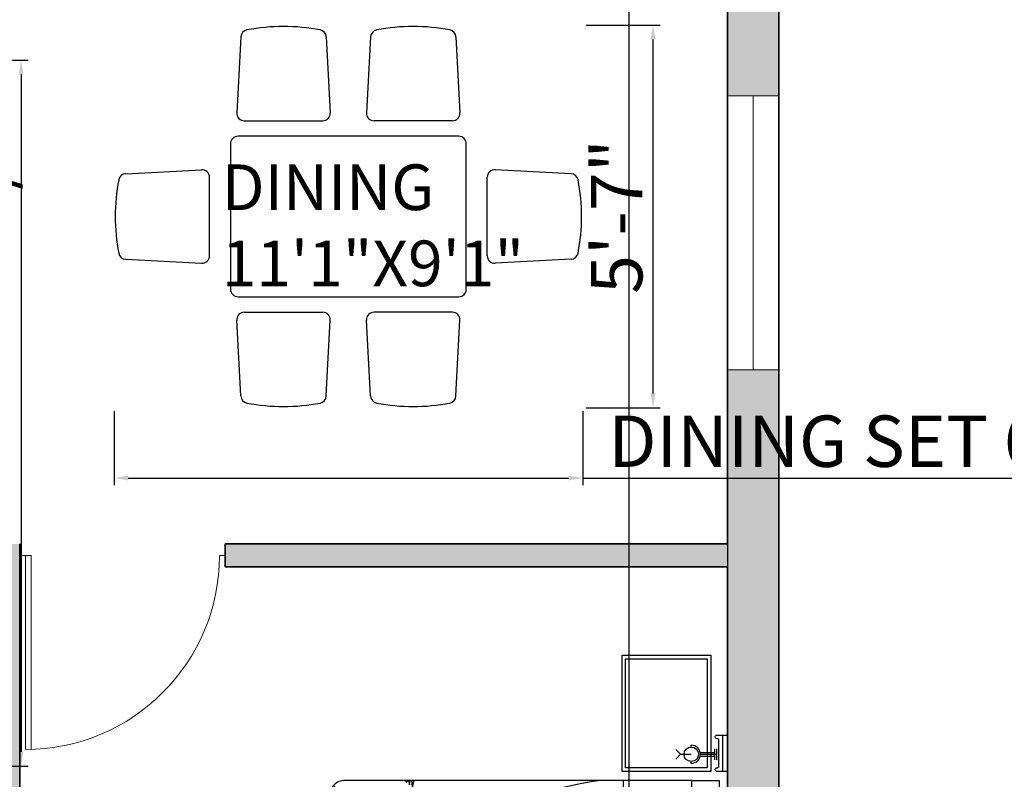
# Model space of a CAD drawing. Units: inches. Extents: x 3592 to 4861, y 1650 to 2243.
# Tile 17 of 30: x 4265 to 4438, y 1870 to 2003. Entities that reach past the tile are written whole.
import ezdxf

# ---------------------------------------------------------------- set-up
doc = ezdxf.new("R2010")
doc.units = ezdxf.units.IN
for name, color, linetype, lineweight in [('A-ANNO-DIMS', 2, 'Continuous', 13), ('A-AREA-IDEN', 7, 'Continuous', 18), ('A-DOOR', 3, 'Continuous', 20), ('A-FURN', 9, 'Continuous', 13), ('A-GLAZ', 4, 'Continuous', 18), ('A-WALL', 7, 'Continuous', 35)]:
    doc.layers.add(name, color=color, linetype=linetype, lineweight=lineweight)
doc.layers.add('A-WALL-PATT', color=252, linetype='Continuous', lineweight=13, true_color=0x939598)
for name, color, linetype in [('CEIL', 4, 'Continuous'), ('ELEC', 4, 'Continuous'), ('FUR', 42, 'Continuous'), ('NOI THAT', 42, 'Continuous'), ('wood', 26, 'Continuous')]:
    doc.layers.add(name, color=color, linetype=linetype)
doc.styles.get("Standard").update_dxf_attribs({"font": 'arial.ttf'})
doc.dimstyles.new('ISO-25', dxfattribs={"dimtxt": 9, "dimasz": 2.5, "dimexe": 1.25, "dimexo": 0.625, "dimtad": 1, "dimlunit": 3, "dimtxsty": 'Standard', "dimcen": 2.5, "dimadec": 0, "dimazin": 0, "dimtfac": 1, "dimtmove": 0, "dimatfit": 3, "dimfxl": 1, "dimarcsym": 0})

# ---------------------------------------------------------------- blocks, each defined once
blk = doc.blocks.new('1')
for p, q in [((3628.27, 1890.86), (3628.27, 1924.86)), ((3629.27, 1890.86), (3629.27, 1924.86)), ((3627.27, 1890.86), (3629.27, 1890.86)), ((3662.27, 1890.86), (3663.27, 1890.86))]:
    blk.add_line(p, q)
blk.add_arc((3628.27, 1890.86), 34, 0, 90)
blk = doc.blocks.new('A$C7568766F')
at = {"layer": 'NOI THAT'}
for p, q in [((647.1, 1940.1), (626, 1538)), ((1100.4, 1940.1), (1121.5, 1538)), ((1334.7, 1940.1), (1313.5, 1538)), ((1787.9, 1940.1), (1809.1, 1538)), ((665.9, 1495.9), (1081.6, 1495.9)), ((1769.2, 1495.9), (1353.5, 1495.9)), ((1802.5, 1413.7), (632.5, 1413.7)), ((592.5, 1373.7), (592.5, 603.7)), ((1842.5, 603.7), (1842.5, 1373.7)), ((37.2, 1215.3), (439.3, 1236.4)), ((2397.9, 1215.3), (1995.8, 1236.4)), ((481.4, 780.8), (481.4, 1196.5)), ((1953.7, 780.8), (1953.7, 1196.5)), ((37.2, 762), (439.3, 740.9)), ((2397.9, 762), (1995.8, 740.9)), ((632.5, 563.7), (1802.5, 563.7)), ((665.9, 481.4), (1081.6, 481.4)), ((1769.2, 481.4), (1353.5, 481.4)), ((647.1, 37.2), (626, 439.3)), ((1100.4, 37.2), (1121.5, 439.3)), ((1334.7, 37.2), (1313.5, 439.3)), ((1787.9, 37.2), (1809.1, 439.3))]:
    blk.add_line(p, q, dxfattribs=at)
for centre, radius, start, end in [((873.8, 970.9), 1025, 79.0754, 100.9246), ((1561.3, 970.9), 1025, 79.0754, 100.9246), ((687.1, 1938), 40, 100.9246, 176.9872), ((1060.4, 1938), 40, 3.0128, 79.0754), ((1374.7, 1938), 40, 100.9246, 176.9872), ((1748, 1938), 40, 3.0128, 79.0754), ((665.9, 1535.9), 40, 176.9872, 270), ((1081.6, 1535.9), 40, 270, 3.0128), ((1353.5, 1535.9), 40, 176.9872, 270), ((1769.2, 1535.9), 40, 270, 3.0128), ((632.5, 1373.7), 40, 90, 180), ((1802.5, 1373.7), 40, 0, 90), ((39.3, 1175.3), 40, 93.0128, 169.0754), ((441.4, 1196.5), 40, 0, 93.0128), ((1993.7, 1196.5), 40, 86.9872, 180), ((2395.8, 1175.3), 40, 10.9246, 86.9872), ((1006.4, 988.7), 1025, 169.0754, 190.9246), ((1428.7, 988.7), 1025, 349.0754, 10.9246), ((39.3, 802), 40, 190.9246, 266.9872), ((2395.8, 802), 40, 273.0128, 349.0754), ((441.4, 780.8), 40, 266.9872, 0), ((1993.7, 780.8), 40, 180, 273.0128), ((632.5, 603.7), 40, 180, 270), ((1802.5, 603.7), 40, 270, 0), ((665.9, 441.4), 40, 90, 183.0128), ((1081.6, 441.4), 40, 356.9872, 90), ((1353.5, 441.4), 40, 90, 183.0128), ((1769.2, 441.4), 40, 356.9872, 90), ((687.1, 39.3), 40, 183.0128, 259.0754), ((1060.4, 39.3), 40, 280.9246, 356.9872), ((1374.7, 39.3), 40, 183.0128, 259.0754), ((1748, 39.3), 40, 280.9246, 356.9872), ((873.8, 1006.4), 1025, 259.0754, 280.9246), ((1561.3, 1006.4), 1025, 259.0754, 280.9246)]:
    blk.add_arc(centre, radius, start, end, dxfattribs=at)
blk = doc.blocks.new('*X20')
at = {"color": 0}
for p, q in [((3155.9, 8182.9), (3155.9, 8182.9)), ((3147.8, 8143.4), (3147.8, 8143.4)), ((3283, 8049.6), (3283, 8049.6)), ((3209.5, 8023.9), (3209.5, 8023.9)), ((3251.6, 7997), (3251.6, 7997)), ((3154.1, 7950.7), (3154.1, 7950.7))]:
    blk.add_line(p, q, dxfattribs=at)
blk = doc.blocks.new('*X19')
at = {"color": 0}
for p, q in [((3155.9, 8182.9), (3155.9, 8182.9)), ((3139.8, 7939.7), (3139.8, 7939.7))]:
    blk.add_line(p, q, dxfattribs=at)
blk = doc.blocks.new('*X18')
at = {"color": 0}
for p, q in [((3155.9, 8182.9), (3155.9, 8182.9)), ((3139.8, 7939.7), (3139.8, 7939.7))]:
    blk.add_line(p, q, dxfattribs=at)
blk = doc.blocks.new('*X17')
at = {"color": 0}
for p, q in [((3163, 7776.2), (3163, 7776.2)), ((3422.2, 7761.3), (3422.2, 7761.3)), ((3236.2, 7675.7), (3236.2, 7675.7)), ((3244.3, 7698.6), (3244.3, 7698.6)), ((3340.3, 7689.4), (3340.3, 7689.4))]:
    blk.add_line(p, q, dxfattribs=at)
blk = doc.blocks.new('BED1')
for p, q in [((0, -1000), (0, 800)), ((150, 800), (0, 800)), ((150, 800), (150, -1000)), ((2058.7, 800), (150, 800)), ((528, 800), (528, -1000)), ((211.8, 614.9), (277.5, 585.4)), ((2537.2, 404.9), (2237.2, 404.9)), ((2187.2, 354.9), (2187.2, -545.1)), ((2587.2, -545.1), (2587.2, 354.9)), ((2566.3, 178.5), (2565.2, 177.4)), ((2582, 188.1), (2565.4, 174.8)), ((2565.4, 174.8), (2585.7, 165.4)), ((2566.3, -296.8), (2565.2, -297.9)), ((2582, -287.1), (2565.4, -300.5)), ((2565.4, -300.5), (2585.7, -309.9)), ((2237.2, -595.1), (2537.2, -595.1)), ((150, -1000), (0, -1000)), ((150, -1000), (2063.5, -1000))]:
    blk.add_line(p, q)
for points in [[(934, 797.9), (930.9, 797.7), (928.3, 797.4), (926.3, 796.9), (924.9, 796.3), (923.8, 795.6), (923.1, 794.8), (922.7, 793.8), (922.5, 792.7), (922.4, 791.5), (922.5, 790.3), (922.6, 789.2), (922.6, 788.3), (922.6, 787.6), (922.4, 787.3), (922, 787.4), (921.4, 787.9), (920.6, 788.9), (919.5, 790.2), (918.4, 791.6), (917.1, 793.1), (915.9, 794.6), (914.6, 796), (913.3, 797.1), (912.2, 797.9), (911.1, 798.3), (910.1, 798.4), (909.2, 798), (908.3, 797.1), (907.5, 795.8), (906.8, 793.9), (906, 791.4), (905.4, 788.5), (904.8, 785.2), (904.2, 781.7), (903.7, 778.4), (903.2, 775.4), (902.8, 772.9), (902.5, 771.3), (902.3, 770.6), (902.1, 771.2), (902, 772.8), (901.8, 775.2), (901.7, 778.1), (901.5, 781.5), (901.2, 785), (900.8, 788.4), (900.2, 791.5), (899.5, 794.1), (898.6, 796.2), (897.6, 797.9), (896.5, 799.2), (895.3, 800), (894.1, 800.5), (893, 800.7), (891.9, 800.5), (890.9, 800.1), (890, 799), (889.1, 797.1), (888.3, 794), (887.6, 789.3), (886.9, 782.9), (886.2, 774.2), (885.5, 763.1), (884.8, 749.5), (884.2, 734.2), (883.6, 718.3), (883, 702.8), (882.5, 688.8), (882, 677.5), (881.7, 669.8), (881.5, 666.9), (881.3, 669.4), (881.3, 676.7), (881.3, 687.8), (881.2, 701.5), (881.1, 716.8), (880.8, 732.6), (880.2, 748), (879.4, 761.8), (878.3, 773.2), (876.9, 782.2), (875.1, 789.2), (872.9, 794.4), (870.3, 798), (869, 799)], [(2150, -913.5), (2150, 723.2)], [(2327.6, 182.3), (2530, 185.9), (2550.8, 181.9), (2561.7, 179), (2566, 176.7), (2566.9, 174.4), (2566.3, 171.9), (2562, 169.2), (2550.3, 166.5), (2527.7, 163.9), (2490.6, 161.8), (2345.5, 160.2), (2317.8, 158.5)], [(494.7, 3.1), (458.9, 95.3)], [(2149.7, -259.9), (2150, -268.4), (2150.1, -274.1), (2150.1, -278.1), (2150, -281.4), (2149.8, -284), (2149.5, -286.1), (2149.1, -287.8), (2148.7, -289), (2148.1, -289.9), (2147.4, -290.5), (2146.6, -290.8), (2145.6, -291), (2144.6, -291), (2143.6, -291), (2142.7, -290.9), (2141.9, -290.9), (2141.4, -290.9), (2141.1, -291), (2141.2, -291.4), (2141.7, -291.9), (2142.5, -292.6), (2143.5, -293.4), (2144.7, -294.4), (2146, -295.4), (2147.2, -296.5), (2148.4, -297.6), (2149.3, -298.6), (2150, -299.6), (2150.3, -300.5), (2150.4, -301.3), (2150, -302.1), (2149.3, -302.8), (2148.2, -303.5), (2146.6, -304.1), (2144.6, -304.7), (2142.1, -305.2), (2139.3, -305.7), (2136.5, -306.2), (2133.7, -306.6), (2131.2, -307), (2129.2, -307.3), (2127.8, -307.6), (2127.3, -307.8), (2127.7, -308), (2129, -308.1), (2131, -308.2), (2133.5, -308.3), (2136.3, -308.5), (2139.2, -308.7), (2142, -309), (2144.6, -309.5), (2146.8, -310.1), (2148.6, -310.9), (2150, -311.7), (2151, -312.7), (2151.7, -313.6), (2152.1, -314.6), (2152.3, -315.6), (2152.2, -316.5), (2151.8, -317.3), (2150.9, -318.1), (2149.3, -318.8), (2146.7, -319.4), (2142.8, -320), (2137.4, -320.6), (2130.2, -321.2), (2121, -321.8), (2109.7, -322.3), (2096.9, -322.9), (2083.6, -323.4), (2070.7, -323.9), (2059.1, -324.3), (2049.6, -324.7), (2043.2, -325), (2040.8, -325.2), (2042.9, -325.3), (2049, -325.3), (2058.2, -325.3), (2069.6, -325.4), (2082.3, -325.5), (2095.6, -325.8), (2108.4, -326.2), (2119.9, -326.8), (2129.4, -327.8), (2136.9, -329), (2142.7, -330.5), (2147, -332.3), (2150, -334.4), (2150.9, -335.6)], [(2246.5, -294.4), (2530, -289.4), (2550.8, -293.4), (2561.7, -296.3), (2566, -298.6), (2566.9, -300.8), (2566.3, -303.4), (2562, -306.1), (2550.3, -308.8), (2527.7, -311.3), (2490.6, -313.5), (2345.5, -315), (2238.6, -321.8)], [(1733.7, -998.3), (1731.1, -998.1), (1729, -997.8), (1727.4, -997.4), (1726.1, -997), (1725.2, -996.4), (1724.7, -995.7), (1724.3, -994.8), (1724.1, -993.9), (1724.1, -992.9), (1724.1, -991.9), (1724.2, -991), (1724.2, -990.2), (1724.2, -989.7), (1724.1, -989.4), (1723.8, -989.5), (1723.2, -990), (1722.5, -990.8), (1721.7, -991.8), (1720.7, -993), (1719.7, -994.3), (1718.6, -995.5), (1717.5, -996.6), (1716.5, -997.6), (1715.5, -998.3), (1714.6, -998.6), (1713.8, -998.6), (1713, -998.3), (1712.3, -997.6), (1711.7, -996.5), (1711, -994.9), (1710.4, -992.9), (1709.9, -990.4), (1709.4, -987.6), (1708.9, -984.8), (1708.5, -982), (1708.1, -979.5), (1707.8, -977.4), (1707.5, -976.1), (1707.3, -975.5), (1707.1, -976), (1707, -977.3), (1706.9, -979.3), (1706.8, -981.8), (1706.7, -984.6), (1706.4, -987.5), (1706.1, -990.3), (1705.6, -992.9), (1705, -995.1), (1704.2, -996.9), (1703.4, -998.3), (1702.4, -999.3), (1701.5, -1000), (1700.5, -1000.4), (1699.6, -1000.6), (1698.7, -1000.4), (1697.8, -1000.1), (1697, -999.2), (1696.3, -997.6), (1695.7, -995), (1695.1, -991.1), (1694.5, -985.7), (1693.9, -978.5), (1693.3, -969.3), (1692.8, -957.9), (1692.2, -945.2), (1691.7, -931.9), (1691.2, -919), (1690.8, -907.4), (1690.4, -897.9), (1690.1, -891.5), (1689.9, -889.1), (1689.8, -891.2), (1689.8, -897.3), (1689.8, -906.5), (1689.7, -917.9), (1689.6, -930.6), (1689.4, -943.8), (1688.9, -956.6), (1688.3, -968.1), (1687.3, -977.6), (1686.1, -985.2), (1684.6, -991), (1682.8, -995.3), (1680.7, -998.3), (1679.6, -999.2)]]:
    blk.add_lwpolyline(points)
for points in [[(205.5, 619.6, 0.267769), (215.1, 582.4, -0.037739), (204.3, 21.8, 0.684696), (236.7, 5.5, -0.060702), (497.2, 0.1, -0.046649), (225.9, 3.1, -1.318436)], [(489.2, 619.6, 0.144019), (207.6, 617.9, 0.248643)], [(497.2, 0.1, 0.021276), (489.2, 619.6, -0.206383), (326.6, 509.4, 0.237198)], [(211.8, 12.8, 0.143972), (361.6, 262.9, 1.292232)], [(886.4, -150, -0.069098), (985, -66.5, 0.658965), (982.1, -48.7, -0.049789), (927.4, -29, -0.103757), (896.6, -5.4, 0.055725), (800.9, 83.3, -0.11866), (782.7, 104.9, 0.016811), (761.6, 143.9, 0.70791), (748.3, 144, -0.16964), (551.9, -96.6, 0.664036), (554, -110.7, 0.023706), (627, -144.7, -0.134834), (683.2, -188, 0.012748), (746.3, -267.4)], [(489.2, -168.2, 0.144019), (207.6, -169.9, 0.248643)], [(969.1, -259.1, 0.263265), (936.3, -236.9, -0.026108), (909.2, -233.2, 0.027613), (945.1, -234.2, -0.089259), (872.7, -120, 0.662242), (857.6, -119.3, -0.162037), (651.8, -332.7, 0.676499), (654, -354.5, -0.160513), (722.9, -401.5, 0.07473), (773.5, -450.3, -0.187721), (845.5, -559.9, 0.70791), (858.8, -561.4, -0.010003), (898.6, -497.3, -0.113819), (947.3, -450.2, 0.099539), (1032.5, -372.4, -0.173425), (1070.9, -346.4, 0.589988), (1076.2, -326.1, 0.137312), (923.9, -245.9, 0.137312)], [(205.5, -168.2, 0.267769), (215.1, -205.4, -0.037739), (204.3, -766, 0.684696), (236.7, -782.3, -0.060702), (497.2, -787.7, -0.046649), (225.9, -784.7, -1.318436)], [(497.2, -787.7, 0.021276), (489.2, -168.2, -0.206383), (326.6, -278.4, 0.237198)], [(1446, -733.4, -0.095039), (652.8, -1001.7)]]:
    blk.add_lwpolyline(points, format="xyb")
for centre, radius, start, end in [((3208.8, 1363.3), 2739.4, 191.8679, 206.3247), ((1138.6, 793.9), 983.2, 294.6078, 358.3033), ((1608.1, 842.5), 496.3, 305.1901, 354.0206), ((2062.7, 713.7), 86.5, 0, 93.5376), ((2237.2, 354.9), 50, 90, 180), ((2321.1, 409.7), 84.5, 185.6196, 217.1396), ((2227.5, 373.5), 32.8, 17.833, 72.8005), ((2546.9, 373.5), 32.8, 107.1995, 162.167), ((2453.3, 409.7), 84.5, 322.8604, 354.3804), ((2537.2, 354.9), 50, 0, 90), ((2098.7, 754.7), 1625, 193.905, 207.8169), ((2201.9, 323.3), 34.8, 50.8413, 114.9586), ((2212.2, 381.5), 36.5, 226.8095, 258.3841), ((2572.5, 323.3), 34.8, 65.0414, 129.1587), ((2562.2, 381.5), 36.5, 281.6159, 313.1905), ((751.8, 88.7), 34.9, 336.8352, 27.7218), ((684.2, 86), 100.3, 353.675, 10.882), ((1074.1, 198.8), 306.1, 197.8602, 241.5122), ((341.4, -277.7), 318.5, 60.7125, 115.009), ((983.7, -79.5), 20.8, 73.7967, 130.4566), ((978.5, -68.6), 14.3, 39.7097, 85.9506), ((602.5, -324), 198.6, 43.2035, 95.0556), ((3208.8, 1363.3), 2739.4, 212.9314, 216.951), ((981.1, -281.8), 131.1, 164.0372, 243.4536), ((980, -379), 163.4, 152.6104, 209.361), ((3208.8, 1363.3), 2739.4, 218.6329, 229.9449), ((2098.7, 754.7), 1625, 226.5887, 246.3156), ((3402.5, -342.9), 1408.5, 182.9917, 205.6819), ((-34.4, -471.2), 376.5, 312.0118, 350.9635), ((2178, -513.5), 33, 286.1827, 338.1386), ((2188.1, -476.2), 73, 269.4513, 322.8027), ((2572.5, -513.6), 34.8, 230.8413, 294.9586), ((2562.2, -571.8), 36.5, 46.8095, 78.3841), ((2237.2, -545.1), 50, 180, 270), ((2271.1, -580.9), 35.8, 148.9055, 197.5541), ((2546.9, -563.8), 32.8, 197.833, 252.8005), ((2453.3, -600), 84.5, 5.6196, 37.1396), ((2537.2, -545.1), 50, 270, 0), ((375.7, -807.4), 128.2, 17.4073, 88.5129), ((341.4, -1065.5), 318.5, 60.7125, 115.009), ((1929.1, -1126), 250.5, 37.8553, 88.4405), ((2063.5, -913.5), 86.5, 270, 0)]:
    blk.add_arc(centre, radius, start, end)
for name in ['*X19', '*X18', '*X20', '*X17']:
    blk.add_blockref(name, (-2425.3, -8101.4))
blk = doc.blocks.new('APLIQ')
at = {"layer": 'ELEC'}
for p, q in [((0, 0.2), (-0.0261, 0.2261)), ((0, 0.2), (0.0261, 0.2261)), ((0, 0.2), (0, 0.14)), ((-0.05, 0.14), (-0.04, 0.14)), ((0.04, 0.14), (0.05, 0.14)), ((-0.01, 0.09), (-0.01, 0.01)), ((0, 0.09), (0, 0)), ((0.01, 0.09), (0.01, 0.01)), ((-0.03, 0.01), (0.03, 0.01)), ((-0.03, 0), (0.03, 0))]:
    blk.add_line(p, q, dxfattribs=at)
blk.add_circle((0, 0.14), 0.04, dxfattribs=at)
blk.add_arc((0, 0.14), 0.05, 180, 0, dxfattribs=at)
blk = doc.blocks.new('A$C68AE1801')
at = {"layer": 'FUR'}
for points in [[(2.5416, 3.18), (2.5416, 2.54), (2.0516, 2.54), (2.0516, 3.18)], [(2.5216, 3.16), (2.5216, 2.56), (2.0716, 2.56), (2.0716, 3.16)], [(2.5416, 0), (2.5416, 0.64), (2.0516, 0.64), (2.0516, 0)], [(2.5216, 0.02), (2.5216, 0.62), (2.0716, 0.62), (2.0716, 0.02)]]:
    blk.add_lwpolyline(points, close=True, dxfattribs=at)
at = {"layer": 'wood'}
for p, q in [((2.6057, 2.74), (2.6057, 2.54)), ((2.6057, 0.44), (2.6057, 0.64))]:
    blk.add_line(p, q, dxfattribs=at)
for points in [[(2.5657, 2.728), (2.5657, 2.732, -0.414214), (2.5737, 2.74), (2.6321, 2.74), (2.6321, 2.54), (2.5737, 2.54, -0.414214), (2.5657, 2.548), (2.5657, 2.552, -0.414214), (2.5737, 2.56), (2.5777, 2.56, 0.414214), (2.5857, 2.568), (2.5857, 2.712, 0.414214), (2.5777, 2.72), (2.5737, 2.72, -0.414214)], [(2.5657, 0.452), (2.5657, 0.448, 0.414214), (2.5737, 0.44), (2.6321, 0.44), (2.6321, 0.64), (2.5737, 0.64, 0.414214), (2.5657, 0.632), (2.5657, 0.628, 0.414214), (2.5737, 0.62), (2.5777, 0.62, -0.414214), (2.5857, 0.612), (2.5857, 0.468, -0.414214), (2.5777, 0.46), (2.5737, 0.46, 0.414214)]]:
    blk.add_lwpolyline(points, format="xyb", close=True, dxfattribs=at)
at = {"layer": 'CEIL', "rotation": 90}
blk.add_blockref('APLIQ', (2.5736, 2.634), dxfattribs=at)
at = {"layer": 'CEIL', "xscale": -1, "rotation": 90}
blk.add_blockref('APLIQ', (2.5736, 0.546), dxfattribs=at)
at = {"layer": 'FUR', "xscale": 0.001, "yscale": 0.001, "zscale": 0.001, "rotation": 180}
blk.add_blockref('BED1', (2.5872, 1.49), dxfattribs=at)
blk = doc.blocks.new('*D158')
at = {"layer": 'A-ANNO-DIMS', "color": 0, "lineweight": -2, "transparency": 16777216}
for p, q in [((4281.9, 1934.46), (4281.9, 1921.52)), ((4364, 1934.46), (4364, 1921.52)), ((4284.4, 1922.77), (4361.5, 1922.77)), ((4364, 1922.77), (4473.66, 1922.77))]:
    blk.add_line(p, q, dxfattribs=at)
at = {"layer": 'A-ANNO-DIMS', "color": 0, "transparency": 16777216}
for points in [[(4284.4, 1923.19), (4284.4, 1922.36), (4281.9, 1922.77)], [(4361.5, 1923.19), (4361.5, 1922.36), (4364, 1922.77)]]:
    blk.add_solid(points, dxfattribs=at)
at = {"layer": 'Defpoints', "color": 0, "transparency": 16777216}
for p in [(4281.9, 1935.09), (4364, 1935.09), (4364, 1922.77)]:
    blk.add_point(p, dxfattribs=at)
at = {"layer": 'A-ANNO-DIMS', "color": 0, "transparency": 16777216, "insert": (4420.08, 1928.05), "char_height": 9, "attachment_point": 5}
blk.add_mtext('DINING SET 6\'-10"', dxfattribs=at)
blk = doc.blocks.new('*D159')
at = {"layer": 'A-ANNO-DIMS', "color": 0, "lineweight": -2, "transparency": 16777216}
for p, q in [((4364.62, 2002.06), (4377.56, 2002.06)), ((4376.31, 1937.59), (4376.31, 1999.56)), ((4364.62, 1935.09), (4377.56, 1935.09))]:
    blk.add_line(p, q, dxfattribs=at)
at = {"layer": 'A-ANNO-DIMS', "color": 0, "transparency": 16777216}
for points in [[(4375.89, 1999.56), (4376.73, 1999.56), (4376.31, 2002.06)], [(4375.89, 1937.59), (4376.73, 1937.59), (4376.31, 1935.09)]]:
    blk.add_solid(points, dxfattribs=at)
at = {"layer": 'Defpoints', "color": 0, "transparency": 16777216}
for p in [(4364, 2002.06), (4376.31, 2002.06), (4364, 1935.09)]:
    blk.add_point(p, dxfattribs=at)
at = {"layer": 'A-ANNO-DIMS', "color": 0, "transparency": 16777216, "insert": (4371.11, 1968.57), "char_height": 9, "attachment_point": 5, "rotation": 90}
blk.add_mtext('5\'-7"', dxfattribs=at)
blk = doc.blocks.new('*D164')
at = {"layer": 'A-ANNO-DIMS', "color": 0, "lineweight": -2, "transparency": 16777216}
for p, q in [((4247.7, 1995.93), (4266.87, 1995.93)), ((4265.62, 1993.43), (4265.62, 1874.82)), ((4247.7, 1872.32), (4266.87, 1872.32))]:
    blk.add_line(p, q, dxfattribs=at)
at = {"layer": 'A-ANNO-DIMS', "color": 0, "transparency": 16777216}
for points in [[(4265.2, 1993.43), (4266.04, 1993.43), (4265.62, 1995.93)], [(4265.2, 1874.82), (4266.04, 1874.82), (4265.62, 1872.32)]]:
    blk.add_solid(points, dxfattribs=at)
at = {"layer": 'Defpoints', "color": 0, "transparency": 16777216}
for p in [(4247.08, 1995.93), (4247.08, 1872.32), (4265.62, 1872.32)]:
    blk.add_point(p, dxfattribs=at)
at = {"layer": 'A-ANNO-DIMS', "color": 0, "transparency": 16777216, "insert": (4260.34, 1934.12), "char_height": 9, "attachment_point": 5, "rotation": 90}
blk.add_mtext('SOFA SET 10\'-3 1/2"', dxfattribs=at)
blk = doc.blocks.new('*D173')
at = {"layer": 'A-ANNO-DIMS', "color": 0, "lineweight": -2, "transparency": 16777216}
for p, q in [((4372.05, 2138.77), (4372.05, 1656.92)), ((4389.37, 2131.59), (4389.37, 1656.92)), ((4374.55, 1658.17), (4386.87, 1658.17)), ((4389.37, 1658.17), (4437.17, 1658.17))]:
    blk.add_line(p, q, dxfattribs=at)
at = {"layer": 'A-ANNO-DIMS', "color": 0, "transparency": 16777216}
for points in [[(4374.55, 1658.59), (4374.55, 1657.75), (4372.05, 1658.17)], [(4386.87, 1658.59), (4386.87, 1657.75), (4389.37, 1658.17)]]:
    blk.add_solid(points, dxfattribs=at)
at = {"layer": 'Defpoints', "color": 0, "transparency": 16777216}
for p in [(4372.05, 2139.4), (4389.37, 2132.22), (4389.37, 1658.17)]:
    blk.add_point(p, dxfattribs=at)
at = {"layer": 'A-ANNO-DIMS', "color": 0, "transparency": 16777216, "insert": (4414.52, 1663.45), "char_height": 9, "attachment_point": 5}
blk.add_mtext('1\'-5 1/2"', dxfattribs=at)

msp = doc.modelspace()

# ---------------------------------------------------------------- hatches: boundary and pattern name
at = {"layer": 'A-WALL-PATT'}
h = msp.add_hatch(color=256, dxfattribs=at)
h.dxf.hatch_style = 1
h.paths.add_polyline_path([(4398.37, 2165.219), (4038.37, 2165.219), (4038.37, 1993.219), (4047.37, 1993.219), (4047.37, 2156.219), (4191.37, 2156.219), (4191.37, 2150.219), (4195.37, 2150.219), (4195.37, 2156.219), (4256.37, 2156.219), (4256.37, 2150.219), (4265.37, 2150.219), (4265.37, 2156.219), (4389.37, 2156.219), (4389.37, 2114.219), (4398.37, 2114.219)])
h.paths.add_polyline_path([(4265.37, 2102.219), (4256.37, 2102.219), (4256.37, 2096.219), (4195.37, 2096.219), (4195.37, 2102.219), (4191.37, 2102.219), (4191.37, 2020.219), (4195.37, 2020.219), (4195.37, 2087.219), (4256.37, 2087.219), (4256.37, 2020.219), (4306.37, 2020.219), (4306.37, 2024.219), (4265.37, 2024.219)], flags=17)
h.paths.add_polyline_path([(4398.37, 2066.219), (4389.37, 2066.219), (4389.37, 2024.219), (4348.37, 2024.219), (4348.37, 2020.219), (4389.37, 2020.219), (4389.37, 1989.719), (4398.37, 1989.719)])
h.paths.add_polyline_path([(4398.37, 1941.719), (4389.37, 1941.719), (4389.37, 1911.219), (4301.37, 1911.219), (4301.37, 1907.219), (4389.37, 1907.219), (4389.37, 1865.219), (4398.37, 1865.219)])
h.paths.add_polyline_path([(4398.37, 1817.219), (4389.37, 1817.219), (4389.37, 1775.219), (4265.37, 1775.219), (4265.37, 1911.219), (4256.37, 1911.219), (4256.37, 1817.219), (4220.87, 1817.219), (4220.87, 1808.219), (4256.37, 1808.219), (4256.37, 1766.219), (4389.37, 1766.219), (4389.37, 1694.219), (4256.37, 1694.219), (4256.37, 1685.219), (4398.37, 1685.219)])
h.paths.add_polyline_path([(4178.87, 1817.219), (4077.37, 1817.219), (4077.37, 1808.219), (4178.87, 1808.219)])
h.paths.add_polyline_path([(4111.37, 2020.219), (4155.37, 2020.219), (4155.37, 2024.219), (4077.37, 2024.219), (4077.37, 2020.219), (4107.37, 2020.219), (4107.37, 1942.219), (4047.37, 1942.219), (4047.37, 1969.219), (4038.37, 1969.219), (4038.37, 1911.219), (4047.37, 1911.219), (4047.37, 1938.219), (4107.37, 1938.219), (4107.37, 1860.219), (4077.37, 1860.219), (4077.37, 1856.219), (4111.37, 1856.219)])
h.paths.add_polyline_path([(4047.37, 1887.219), (4038.37, 1887.219), (4038.37, 1685.219), (4152.37, 1685.219), (4152.37, 1715.219), (4143.37, 1715.219), (4143.37, 1694.219), (4047.37, 1694.219)])
h.paths.add_polyline_path([(4152.37, 1772.219), (4143.37, 1772.219), (4143.37, 1751.219), (4152.37, 1751.219)], flags=17)

# ---------------------------------------------------------------- linework, layer by layer
at = {"layer": 'A-GLAZ'}
for p, q in [((4389.37, 1989.719), (4398.37, 1989.719)), ((4393.87, 1989.719), (4393.87, 1941.719)), ((4389.37, 1941.719), (4398.37, 1941.719))]:
    msp.add_line(p, q, dxfattribs=at)
at = {"layer": 'A-WALL'}
for p, q in [((4398.37, 2165.219), (4398.37, 1685.219)), ((4389.37, 2020.219), (4389.37, 1911.219)), ((4265.37, 1911.219), (4265.37, 1775.219)), ((4301.37, 1911.219), (4301.37, 1907.219)), ((4389.37, 1911.219), (4301.37, 1911.219)), ((4389.37, 1907.219), (4301.37, 1907.219)), ((4389.37, 1907.219), (4389.37, 1775.219))]:
    msp.add_line(p, q, dxfattribs=at)

# ---------------------------------------------------------------- block references
at = {"layer": 'A-DOOR', "xscale": -1, "rotation": 180}
msp.add_blockref('1', (638.102, 3800.083), dxfattribs=at)
at = {"layer": 'A-FURN'}
for name, p, xscale, yscale, zscale in [('A$C7568766F', (4282.716, 1935.907), 0.0330425380115637, 0.0330425380115637, 0.0330425380115637), ('A$C68AE1801', (4305.708, 1790.711), 31.7658940618111, 31.7658940618111, 31.7658940618111)]:
    msp.add_blockref(name, p, dxfattribs=dict(at, xscale=xscale, yscale=yscale, zscale=zscale))

# ---------------------------------------------------------------- texts
at = {"layer": 'A-AREA-IDEN', "insert": (4300.765, 1977.695), "char_height": 8, "attachment_point": 1}
msp.add_mtext_dynamic_manual_height_columns('DINING\\P11\'1"X9\'1"', width=121.44943, gutter_width=12.5, heights=[0], dxfattribs=at)

# ---------------------------------------------------------------- dimensions: what is measured, and where the dimension line sits
at = {"layer": 'A-ANNO-DIMS'}
dim = msp.add_linear_dim(base=(4389.37, 1658.169), p1=(4372.046, 2139.399), p2=(4389.37, 2132.219), dimstyle='ISO-25', override={"dimdec": 1, "dimlfac": 1, "dimrnd": 0, "dimzin": 1, "dimdsep": 46, "dimlunit": 4, "dimfrac": 2}, dxfattribs=at)
dim.commit()
dim.dimension.update_dxf_attribs({"geometry": '*D173', "text_midpoint": (4414.519, 1663.447)})
dim = msp.add_linear_dim(base=(4376.31, 2002.061), p1=(4363.996, 1935.089), p2=(4363.996, 2002.061), angle=90, dimstyle='ISO-25', override={"dimdec": 1, "dimlfac": 1, "dimrnd": 0, "dimzin": 1, "dimdsep": 46, "dimlunit": 4, "dimfrac": 2}, dxfattribs=at)
dim.commit()
dim.dimension.update_dxf_attribs({"geometry": '*D159', "text_midpoint": (4371.109, 1968.575)})
dim = msp.add_linear_dim(base=(4265.62, 1872.318), p1=(4247.079, 1995.926), p2=(4247.079, 1872.318), angle=270, text='SOFA SET <>', dimstyle='ISO-25', override={"dimdec": 1, "dimlfac": 1, "dimrnd": 0, "dimzin": 1, "dimdsep": 46, "dimlunit": 4, "dimfrac": 2}, dxfattribs=at)
dim.commit()
dim.dimension.update_dxf_attribs({"geometry": '*D164', "text_midpoint": (4260.336, 1934.122)})
dim = msp.add_linear_dim(base=(4363.996, 1922.774), p1=(4281.898, 1935.089), p2=(4363.996, 1935.089), text='DINING SET <>', dimstyle='ISO-25', override={"dimdec": 1, "dimlfac": 1, "dimrnd": 0, "dimzin": 1, "dimdsep": 46, "dimlunit": 4, "dimfrac": 2}, dxfattribs=at)
dim.commit()
dim.dimension.update_dxf_attribs({"geometry": '*D158', "text_midpoint": (4420.077, 1928.052)})

doc.saveas('drawing.dxf')
